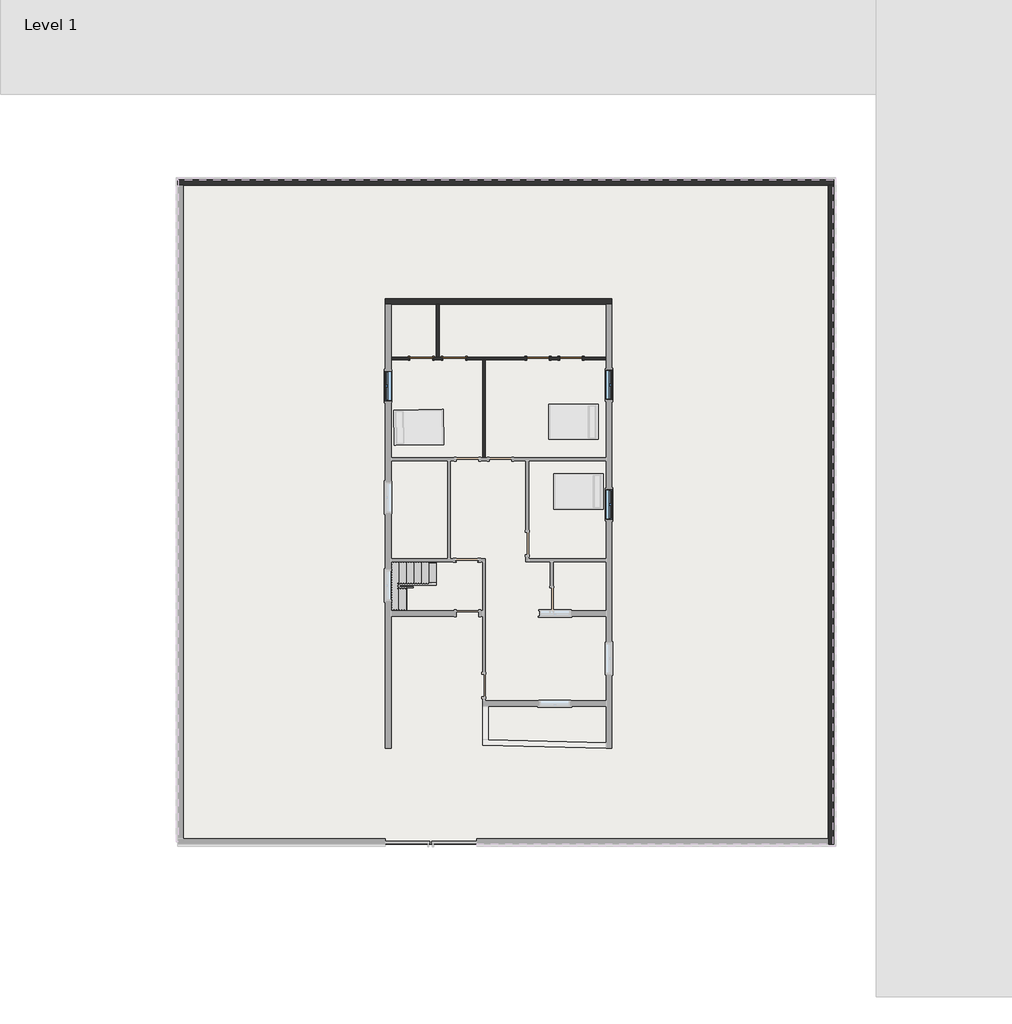
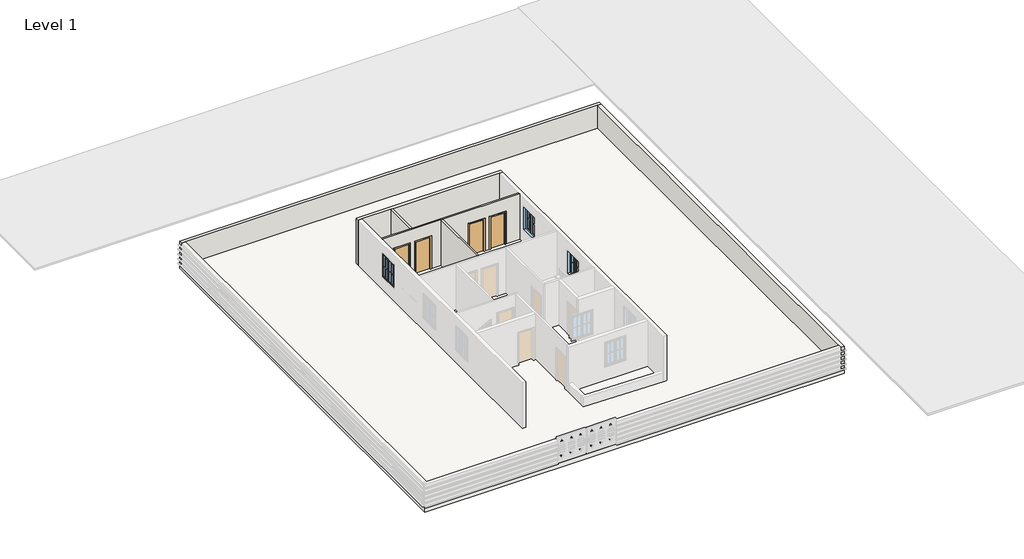
# One storey, part 2 of 3: 6 walls, 4 doors, 3 windows, 1 railing, 1 slab, 1 stair flight.
"""IFC4 building model written with IfcOpenShell, lengths in millimetres."""

from ifc_helpers import new_model, si_unit, frame, origin, origin_with_axes, place, context, project, spatial, polyline, outline, extrude, faceted_brep, transform, mapped, element, save
from components import door_e5f9f3c4, door_305aa2a5, stair_flight_da774960, window_8377141f

model = new_model("IFC4")

# Units and contexts
model_context = context("Model", 3, world=origin())
ifc_project = project(units=[si_unit("LENGTHUNIT", "METRE", prefix="MILLI")], contexts=[model_context])

# Site, building, storey
site = spatial("IfcSite", under=ifc_project)
building = spatial("IfcBuilding", under=site)
storey = spatial("IfcBuildingStorey", under=building, Name="Level 1", Elevation=0.0)

# Doors
placement = place(None, origin())
door_shape = door_e5f9f3c4(model_context)
element("IfcDoor", 1, ObjectType="Single-Flush : 36\" x 84\"", at=placement, inside=storey, context=model_context, shape_type="MappedRepresentation", body=[
    mapped(door_shape, transform((7442.2, 11550.65, 0.0), x_axis=(1.0, 0.0, 0.0), y_axis=(0.0, 1.0, 0.0), z_axis=(0.0, 0.0, 1.0))),
])
element("IfcDoor", 2, ObjectType="Single-Flush : 36\" x 84\"", at=placement, inside=storey, context=model_context, shape_type="MappedRepresentation", body=[
    mapped(door_shape, transform((2717.8, 11550.65, 0.0), x_axis=(1.0, 0.0, 0.0), y_axis=(0.0, 1.0, 0.0), z_axis=(0.0, 0.0, 1.0))),
])
door_2_shape = door_305aa2a5(model_context)
element("IfcDoor", 3, ObjectType="Single-Flush : 36\" x 84\"", at=placement, inside=storey, context=model_context, shape_type="MappedRepresentation", body=[
    mapped(door_2_shape, transform((4051.3, 11550.65, 0.0), x_axis=(-1.0, 0.0, 0.0), y_axis=(0.0, -1.0, 0.0), z_axis=(0.0, 0.0, 1.0))),
])
element("IfcDoor", 4, ObjectType="Single-Flush : 36\" x 84\"", at=placement, inside=storey, context=model_context, shape_type="MappedRepresentation", body=[
    mapped(door_2_shape, transform((8775.7, 11550.65, 0.0), x_axis=(-1.0, 0.0, 0.0), y_axis=(0.0, -1.0, 0.0), z_axis=(0.0, 0.0, 1.0))),
])

# Railing
element("IfcRailing", 5, ObjectType="Handrail - Rectangular", at=placement, inside=storey, context=model_context, shape_type="SolidModel", body=[
    faceted_brep([(3327.4, 3289.3, 1083.7333333), (3327.4, 3289.3, 1025.620221), (3327.4, 3340.1, 1025.620221), (3327.4, 3340.1, 1083.7333333), (1803.4, 3289.3, 1930.4), (1790.2363978, 3289.3, 1879.6), (1790.2363978, 3340.1, 1879.6), (1803.4, 3340.1, 1930.4), (1549.4, 3289.3, 1930.4), (1549.4, 3289.3, 1879.6), (1498.6, 3340.1, 1879.6), (1498.6, 3340.1, 1930.4), (1549.4, 1485.9, 1930.4), (1549.4, 1435.1, 1879.6), (1498.6, 1435.1, 1879.6), (1498.6, 1485.9, 1930.4), (1549.4, 1485.9, 2000.9555556), (1549.4, 1435.1, 1950.1555556), (1498.6, 1435.1, 1950.1555556), (1498.6, 1485.9, 2000.9555556), (1549.4, 1409.7, 2000.9555556), (1549.4, 1409.7, 1950.1555556), (1498.6, 1358.9, 1950.1555556), (1498.6, 1358.9, 2000.9555556), (1625.6, 1409.7, 2000.9555556), (1638.7636022, 1409.7, 1950.1555556), (1638.7636022, 1358.9, 1950.1555556), (1625.6, 1358.9, 2000.9555556), (3022.6, 1409.7, 2777.0666667), (3022.6, 1358.9, 2777.0666667), (3022.6, 1358.9, 2718.9535543), (3022.6, 1409.7, 2718.9535543)], [[[0, 1, 2, 3]], [[1, 0, 4, 5]], [[2, 1, 5, 6]], [[3, 2, 6, 7]], [[0, 3, 7, 4]], [[5, 4, 8, 9]], [[6, 5, 9, 10]], [[7, 6, 10, 11]], [[4, 7, 11, 8]], [[9, 8, 12, 13]], [[10, 9, 13, 14]], [[11, 10, 14, 15]], [[8, 11, 15, 12]], [[13, 12, 16, 17]], [[14, 13, 17, 18]], [[15, 14, 18, 19]], [[12, 15, 19, 16]], [[17, 16, 20, 21]], [[18, 17, 21, 22]], [[19, 18, 22, 23]], [[16, 19, 23, 20]], [[21, 20, 24, 25]], [[22, 21, 25, 26]], [[23, 22, 26, 27]], [[20, 23, 27, 24]], [[28, 29, 30, 31]], [[25, 24, 28, 31]], [[26, 25, 31, 30]], [[27, 26, 30, 29]], [[24, 27, 29, 28]]]),
    extrude(outline(polyline([(2681.9118876, 2955.925), (2671.3285543, 2936.875), (1693.3333333, 2936.875), (1693.3333333, 2955.925), (2681.9118876, 2955.925)])), frame((0.0, 1374.775, 0.0), z_axis=(0.0, 1.0, 0.0), x_axis=(0.0, 0.0, 1.0)), (0.0, 0.0, 1.0), 19.05),
    extrude(outline(polyline([(2625.4674432, 2854.325), (2614.8841099, 2835.275), (1693.3333333, 2835.275), (1693.3333333, 2854.325), (2625.4674432, 2854.325)])), frame((0.0, 1374.775, 0.0), z_axis=(0.0, 1.0, 0.0), x_axis=(0.0, 0.0, 1.0)), (0.0, 0.0, 1.0), 19.05),
    extrude(outline(polyline([(2569.0229988, 2752.725), (2558.4396654, 2733.675), (1693.3333333, 2733.675), (1693.3333333, 2752.725), (2569.0229988, 2752.725)])), frame((0.0, 1374.775, 0.0), z_axis=(0.0, 1.0, 0.0), x_axis=(0.0, 0.0, 1.0)), (0.0, 0.0, 1.0), 19.05),
    extrude(outline(polyline([(2512.5785543, 2651.125), (2501.995221, 2632.075), (1524.0, 2632.075), (1524.0, 2651.125), (2512.5785543, 2651.125)])), frame((0.0, 1374.775, 0.0), z_axis=(0.0, 1.0, 0.0), x_axis=(0.0, 0.0, 1.0)), (0.0, 0.0, 1.0), 19.05),
    extrude(outline(polyline([(2456.1341099, 2549.525), (2445.5507765, 2530.475), (1524.0, 2530.475), (1524.0, 2549.525), (2456.1341099, 2549.525)])), frame((0.0, 1374.775, 0.0), z_axis=(0.0, 1.0, 0.0), x_axis=(0.0, 0.0, 1.0)), (0.0, 0.0, 1.0), 19.05),
    extrude(outline(polyline([(2399.6896654, 2447.925), (2389.1063321, 2428.875), (1524.0, 2428.875), (1524.0, 2447.925), (2399.6896654, 2447.925)])), frame((0.0, 1374.775, 0.0), z_axis=(0.0, 1.0, 0.0), x_axis=(0.0, 0.0, 1.0)), (0.0, 0.0, 1.0), 19.05),
    extrude(outline(polyline([(2343.245221, 2346.325), (2332.6618876, 2327.275), (1354.6666667, 2327.275), (1354.6666667, 2346.325), (2343.245221, 2346.325)])), frame((0.0, 1374.775, 0.0), z_axis=(0.0, 1.0, 0.0), x_axis=(0.0, 0.0, 1.0)), (0.0, 0.0, 1.0), 19.05),
    extrude(outline(polyline([(2286.8007765, 2244.725), (2276.2174432, 2225.675), (1354.6666667, 2225.675), (1354.6666667, 2244.725), (2286.8007765, 2244.725)])), frame((0.0, 1374.775, 0.0), z_axis=(0.0, 1.0, 0.0), x_axis=(0.0, 0.0, 1.0)), (0.0, 0.0, 1.0), 19.05),
    extrude(outline(polyline([(2230.3563321, 2143.125), (2219.7729988, 2124.075), (1354.6666667, 2124.075), (1354.6666667, 2143.125), (2230.3563321, 2143.125)])), frame((0.0, 1374.775, 0.0), z_axis=(0.0, 1.0, 0.0), x_axis=(0.0, 0.0, 1.0)), (0.0, 0.0, 1.0), 19.05),
    extrude(outline(polyline([(2173.9118876, 2041.525), (2163.3285543, 2022.475), (1185.3333333, 2022.475), (1185.3333333, 2041.525), (2173.9118876, 2041.525)])), frame((0.0, 1374.775, 0.0), z_axis=(0.0, 1.0, 0.0), x_axis=(0.0, 0.0, 1.0)), (0.0, 0.0, 1.0), 19.05),
    extrude(outline(polyline([(2117.4674432, 1939.925), (2106.8841099, 1920.875), (1185.3333333, 1920.875), (1185.3333333, 1939.925), (2117.4674432, 1939.925)])), frame((0.0, 1374.775, 0.0), z_axis=(0.0, 1.0, 0.0), x_axis=(0.0, 0.0, 1.0)), (0.0, 0.0, 1.0), 19.05),
    extrude(outline(polyline([(2061.0229988, 1838.325), (2050.4396654, 1819.275), (1185.3333333, 1819.275), (1185.3333333, 1838.325), (2061.0229988, 1838.325)])), frame((0.0, 1374.775, 0.0), z_axis=(0.0, 1.0, 0.0), x_axis=(0.0, 0.0, 1.0)), (0.0, 0.0, 1.0), 19.05),
    extrude(outline(polyline([(2004.5785543, 1736.725), (1993.995221, 1717.675), (1016.0, 1717.675), (1016.0, 1736.725), (2004.5785543, 1736.725)])), frame((0.0, 1374.775, 0.0), z_axis=(0.0, 1.0, 0.0), x_axis=(0.0, 0.0, 1.0)), (0.0, 0.0, 1.0), 19.05),
    extrude(outline(polyline([(1948.1341099, 1635.125), (1937.5507765, 1616.075), (1016.0, 1616.075), (1016.0, 1635.125), (1948.1341099, 1635.125)])), frame((0.0, 1374.775, 0.0), z_axis=(0.0, 1.0, 0.0), x_axis=(0.0, 0.0, 1.0)), (0.0, 0.0, 1.0), 19.05),
    extrude(outline(polyline([(1514.475, 1495.425), (1533.525, 1495.425), (1533.525, 1476.375), (1514.475, 1476.375), (1514.475, 1495.425)])), frame((0.0, 0.0, 1016.0), z_axis=(0.0, 0.0, 1.0), x_axis=(1.0, 0.0, 0.0)), (0.0, 0.0, 1.0), 863.6),
    extrude(outline(polyline([(1514.475, 1597.025), (1533.525, 1597.025), (1533.525, 1577.975), (1514.475, 1577.975), (1514.475, 1597.025)])), frame((0.0, 0.0, 1016.0), z_axis=(0.0, 0.0, 1.0), x_axis=(1.0, 0.0, 0.0)), (0.0, 0.0, 1.0), 863.6),
    extrude(outline(polyline([(1514.475, 1698.625), (1533.525, 1698.625), (1533.525, 1679.575), (1514.475, 1679.575), (1514.475, 1698.625)])), frame((0.0, 0.0, 1016.0), z_axis=(0.0, 0.0, 1.0), x_axis=(1.0, 0.0, 0.0)), (0.0, 0.0, 1.0), 863.6),
    extrude(outline(polyline([(1514.475, 1800.225), (1533.525, 1800.225), (1533.525, 1781.175), (1514.475, 1781.175), (1514.475, 1800.225)])), frame((0.0, 0.0, 1016.0), z_axis=(0.0, 0.0, 1.0), x_axis=(1.0, 0.0, 0.0)), (0.0, 0.0, 1.0), 863.6),
    extrude(outline(polyline([(1514.475, 1901.825), (1533.525, 1901.825), (1533.525, 1882.775), (1514.475, 1882.775), (1514.475, 1901.825)])), frame((0.0, 0.0, 1016.0), z_axis=(0.0, 0.0, 1.0), x_axis=(1.0, 0.0, 0.0)), (0.0, 0.0, 1.0), 863.6),
    extrude(outline(polyline([(1514.475, 2003.425), (1533.525, 2003.425), (1533.525, 1984.375), (1514.475, 1984.375), (1514.475, 2003.425)])), frame((0.0, 0.0, 1016.0), z_axis=(0.0, 0.0, 1.0), x_axis=(1.0, 0.0, 0.0)), (0.0, 0.0, 1.0), 863.6),
    extrude(outline(polyline([(1514.475, 2105.025), (1533.525, 2105.025), (1533.525, 2085.975), (1514.475, 2085.975), (1514.475, 2105.025)])), frame((0.0, 0.0, 1016.0), z_axis=(0.0, 0.0, 1.0), x_axis=(1.0, 0.0, 0.0)), (0.0, 0.0, 1.0), 863.6),
    extrude(outline(polyline([(1514.475, 2206.625), (1533.525, 2206.625), (1533.525, 2187.575), (1514.475, 2187.575), (1514.475, 2206.625)])), frame((0.0, 0.0, 1016.0), z_axis=(0.0, 0.0, 1.0), x_axis=(1.0, 0.0, 0.0)), (0.0, 0.0, 1.0), 863.6),
    extrude(outline(polyline([(1514.475, 2308.225), (1533.525, 2308.225), (1533.525, 2289.175), (1514.475, 2289.175), (1514.475, 2308.225)])), frame((0.0, 0.0, 1016.0), z_axis=(0.0, 0.0, 1.0), x_axis=(1.0, 0.0, 0.0)), (0.0, 0.0, 1.0), 863.6),
    extrude(outline(polyline([(1514.475, 2409.825), (1533.525, 2409.825), (1533.525, 2390.775), (1514.475, 2390.775), (1514.475, 2409.825)])), frame((0.0, 0.0, 1016.0), z_axis=(0.0, 0.0, 1.0), x_axis=(1.0, 0.0, 0.0)), (0.0, 0.0, 1.0), 863.6),
    extrude(outline(polyline([(1514.475, 2511.425), (1533.525, 2511.425), (1533.525, 2492.375), (1514.475, 2492.375), (1514.475, 2511.425)])), frame((0.0, 0.0, 1016.0), z_axis=(0.0, 0.0, 1.0), x_axis=(1.0, 0.0, 0.0)), (0.0, 0.0, 1.0), 863.6),
    extrude(outline(polyline([(1514.475, 2613.025), (1533.525, 2613.025), (1533.525, 2593.975), (1514.475, 2593.975), (1514.475, 2613.025)])), frame((0.0, 0.0, 1016.0), z_axis=(0.0, 0.0, 1.0), x_axis=(1.0, 0.0, 0.0)), (0.0, 0.0, 1.0), 863.6),
    extrude(outline(polyline([(1514.475, 2714.625), (1533.525, 2714.625), (1533.525, 2695.575), (1514.475, 2695.575), (1514.475, 2714.625)])), frame((0.0, 0.0, 1016.0), z_axis=(0.0, 0.0, 1.0), x_axis=(1.0, 0.0, 0.0)), (0.0, 0.0, 1.0), 863.6),
    extrude(outline(polyline([(1514.475, 2816.225), (1533.525, 2816.225), (1533.525, 2797.175), (1514.475, 2797.175), (1514.475, 2816.225)])), frame((0.0, 0.0, 1016.0), z_axis=(0.0, 0.0, 1.0), x_axis=(1.0, 0.0, 0.0)), (0.0, 0.0, 1.0), 863.6),
    extrude(outline(polyline([(1514.475, 2917.825), (1533.525, 2917.825), (1533.525, 2898.775), (1514.475, 2898.775), (1514.475, 2917.825)])), frame((0.0, 0.0, 1016.0), z_axis=(0.0, 0.0, 1.0), x_axis=(1.0, 0.0, 0.0)), (0.0, 0.0, 1.0), 863.6),
    extrude(outline(polyline([(1514.475, 3019.425), (1533.525, 3019.425), (1533.525, 3000.375), (1514.475, 3000.375), (1514.475, 3019.425)])), frame((0.0, 0.0, 1016.0), z_axis=(0.0, 0.0, 1.0), x_axis=(1.0, 0.0, 0.0)), (0.0, 0.0, 1.0), 863.6),
    extrude(outline(polyline([(1514.475, 3121.025), (1533.525, 3121.025), (1533.525, 3101.975), (1514.475, 3101.975), (1514.475, 3121.025)])), frame((0.0, 0.0, 1016.0), z_axis=(0.0, 0.0, 1.0), x_axis=(1.0, 0.0, 0.0)), (0.0, 0.0, 1.0), 863.6),
    extrude(outline(polyline([(1514.475, 3222.625), (1533.525, 3222.625), (1533.525, 3203.575), (1514.475, 3203.575), (1514.475, 3222.625)])), frame((0.0, 0.0, 1016.0), z_axis=(0.0, 0.0, 1.0), x_axis=(1.0, 0.0, 0.0)), (0.0, 0.0, 1.0), 863.6),
    extrude(outline(polyline([(1609.725, 3324.225), (1609.725, 3305.175), (1590.675, 3305.175), (1590.675, 3324.225), (1609.725, 3324.225)])), frame((0.0, 0.0, 1016.0), z_axis=(0.0, 0.0, 1.0), x_axis=(1.0, 0.0, 0.0)), (0.0, 0.0, 1.0), 863.6),
    extrude(outline(polyline([(1711.325, 3324.225), (1711.325, 3305.175), (1692.275, 3305.175), (1692.275, 3324.225), (1711.325, 3324.225)])), frame((0.0, 0.0, 1016.0), z_axis=(0.0, 0.0, 1.0), x_axis=(1.0, 0.0, 0.0)), (0.0, 0.0, 1.0), 863.6),
    extrude(outline(polyline([(1866.995221, 1812.925), (1877.5785543, 1793.875), (1016.0, 1793.875), (1016.0, 1812.925), (1866.995221, 1812.925)])), frame((0.0, 3305.175, 0.0), z_axis=(0.0, 1.0, 0.0), x_axis=(0.0, 0.0, 1.0)), (0.0, 0.0, 1.0), 19.05),
    extrude(outline(polyline([(1810.5507765, 1914.525), (1821.1341099, 1895.475), (846.6666667, 1895.475), (846.6666667, 1914.525), (1810.5507765, 1914.525)])), frame((0.0, 3305.175, 0.0), z_axis=(0.0, 1.0, 0.0), x_axis=(0.0, 0.0, 1.0)), (0.0, 0.0, 1.0), 19.05),
    extrude(outline(polyline([(1754.1063321, 2016.125), (1764.6896654, 1997.075), (846.6666667, 1997.075), (846.6666667, 2016.125), (1754.1063321, 2016.125)])), frame((0.0, 3305.175, 0.0), z_axis=(0.0, 1.0, 0.0), x_axis=(0.0, 0.0, 1.0)), (0.0, 0.0, 1.0), 19.05),
    extrude(outline(polyline([(1697.6618876, 2117.725), (1708.245221, 2098.675), (846.6666667, 2098.675), (846.6666667, 2117.725), (1697.6618876, 2117.725)])), frame((0.0, 3305.175, 0.0), z_axis=(0.0, 1.0, 0.0), x_axis=(0.0, 0.0, 1.0)), (0.0, 0.0, 1.0), 19.05),
    extrude(outline(polyline([(1641.2174432, 2219.325), (1651.8007765, 2200.275), (677.3333333, 2200.275), (677.3333333, 2219.325), (1641.2174432, 2219.325)])), frame((0.0, 3305.175, 0.0), z_axis=(0.0, 1.0, 0.0), x_axis=(0.0, 0.0, 1.0)), (0.0, 0.0, 1.0), 19.05),
    extrude(outline(polyline([(1584.7729988, 2320.925), (1595.3563321, 2301.875), (677.3333333, 2301.875), (677.3333333, 2320.925), (1584.7729988, 2320.925)])), frame((0.0, 3305.175, 0.0), z_axis=(0.0, 1.0, 0.0), x_axis=(0.0, 0.0, 1.0)), (0.0, 0.0, 1.0), 19.05),
    extrude(outline(polyline([(1528.3285543, 2422.525), (1538.9118876, 2403.475), (677.3333333, 2403.475), (677.3333333, 2422.525), (1528.3285543, 2422.525)])), frame((0.0, 3305.175, 0.0), z_axis=(0.0, 1.0, 0.0), x_axis=(0.0, 0.0, 1.0)), (0.0, 0.0, 1.0), 19.05),
    extrude(outline(polyline([(1471.8841099, 2524.125), (1482.4674432, 2505.075), (508.0, 2505.075), (508.0, 2524.125), (1471.8841099, 2524.125)])), frame((0.0, 3305.175, 0.0), z_axis=(0.0, 1.0, 0.0), x_axis=(0.0, 0.0, 1.0)), (0.0, 0.0, 1.0), 19.05),
    extrude(outline(polyline([(1415.4396654, 2625.725), (1426.0229988, 2606.675), (508.0, 2606.675), (508.0, 2625.725), (1415.4396654, 2625.725)])), frame((0.0, 3305.175, 0.0), z_axis=(0.0, 1.0, 0.0), x_axis=(0.0, 0.0, 1.0)), (0.0, 0.0, 1.0), 19.05),
    extrude(outline(polyline([(1358.995221, 2727.325), (1369.5785543, 2708.275), (508.0, 2708.275), (508.0, 2727.325), (1358.995221, 2727.325)])), frame((0.0, 3305.175, 0.0), z_axis=(0.0, 1.0, 0.0), x_axis=(0.0, 0.0, 1.0)), (0.0, 0.0, 1.0), 19.05),
    extrude(outline(polyline([(1302.5507765, 2828.925), (1313.1341099, 2809.875), (338.6666667, 2809.875), (338.6666667, 2828.925), (1302.5507765, 2828.925)])), frame((0.0, 3305.175, 0.0), z_axis=(0.0, 1.0, 0.0), x_axis=(0.0, 0.0, 1.0)), (0.0, 0.0, 1.0), 19.05),
    extrude(outline(polyline([(1246.1063321, 2930.525), (1256.6896654, 2911.475), (338.6666667, 2911.475), (338.6666667, 2930.525), (1246.1063321, 2930.525)])), frame((0.0, 3305.175, 0.0), z_axis=(0.0, 1.0, 0.0), x_axis=(0.0, 0.0, 1.0)), (0.0, 0.0, 1.0), 19.05),
    extrude(outline(polyline([(1189.6618876, 3032.125), (1200.245221, 3013.075), (338.6666667, 3013.075), (338.6666667, 3032.125), (1189.6618876, 3032.125)])), frame((0.0, 3305.175, 0.0), z_axis=(0.0, 1.0, 0.0), x_axis=(0.0, 0.0, 1.0)), (0.0, 0.0, 1.0), 19.05),
    extrude(outline(polyline([(1133.2174432, 3133.725), (1143.8007765, 3114.675), (169.3333333, 3114.675), (169.3333333, 3133.725), (1133.2174432, 3133.725)])), frame((0.0, 3305.175, 0.0), z_axis=(0.0, 1.0, 0.0), x_axis=(0.0, 0.0, 1.0)), (0.0, 0.0, 1.0), 19.05),
    extrude(outline(polyline([(1076.7729988, 3235.325), (1087.3563321, 3216.275), (169.3333333, 3216.275), (169.3333333, 3235.325), (1076.7729988, 3235.325)])), frame((0.0, 3305.175, 0.0), z_axis=(0.0, 1.0, 0.0), x_axis=(0.0, 0.0, 1.0)), (0.0, 0.0, 1.0), 19.05),
    extrude(outline(polyline([(1514.475, 1393.825), (1533.525, 1393.825), (1533.525, 1374.775), (1514.475, 1374.775), (1514.475, 1393.825)])), frame((0.0, 0.0, 1016.0), z_axis=(0.0, 0.0, 1.0), x_axis=(1.0, 0.0, 0.0)), (0.0, 0.0, 1.0), 934.1555556),
    extrude(outline(polyline([(1533.525, 3324.225), (1533.525, 3305.175), (1514.475, 3305.175), (1514.475, 3324.225), (1533.525, 3324.225)])), frame((0.0, 0.0, 1016.0), z_axis=(0.0, 0.0, 1.0), x_axis=(1.0, 0.0, 0.0)), (0.0, 0.0, 1.0), 863.6),
    extrude(outline(polyline([(2718.9535543, 3022.6), (2708.370221, 3003.55), (1693.3333333, 3003.55), (1693.3333333, 3022.6), (2718.9535543, 3022.6)])), frame((0.0, 1374.775, 0.0), z_axis=(0.0, 1.0, 0.0), x_axis=(0.0, 0.0, 1.0)), (0.0, 0.0, 1.0), 19.05),
    extrude(outline(polyline([(1025.620221, 3327.4), (1036.2035543, 3308.35), (169.3333333, 3308.35), (169.3333333, 3327.4), (1025.620221, 3327.4)])), frame((0.0, 3305.175, 0.0), z_axis=(0.0, 1.0, 0.0), x_axis=(0.0, 0.0, 1.0)), (0.0, 0.0, 1.0), 19.05),
])

# Slab
element("IfcSlab", 6, ObjectType="Generic - 12\"", at=placement, inside=storey, context=model_context, shape_type="SweptSolid", body=[
    extrude(outline(polyline([(19396.129742, 18780.9634228), (19396.129742, -8092.2365772), (-7121.470258, -8092.2365772), (-7121.470258, 18780.9634228), (19396.129742, 18780.9634228)])), frame((0.0, 0.0, -304.8), z_axis=(0.0, 0.0, 1.0), x_axis=(1.0, 0.0, 0.0)), (0.0, 0.0, 1.0), 304.8),
])

# Stair flight
stair_flight_shape = stair_flight_da774960(model_context)
element("IfcStairFlight", 7, ObjectType="2\" Tread 1\" Nosing 1/4\" Riser", at=placement, inside=storey, context=model_context, shape_type="MappedRepresentation", body=[
    mapped(stair_flight_shape, transform((0.0, 0.0, 0.0), x_axis=(1.0, 0.0, 0.0), y_axis=(0.0, 1.0, 0.0), z_axis=(0.0, 0.0, 1.0))),
])

# Walls
element("IfcWall", 8, ObjectType="Generic - 5\"", at=placement, inside=storey, context=model_context, shape_type="SweptSolid", body=[
    extrude(outline(polyline([(3327.4, 11607.8), (3327.4, 13741.4), (3441.7, 13741.4), (3441.7, 11607.8), (3327.4, 11607.8)])), origin_with_axes(), (0.0, 0.0, 1.0), 3048.0),
])
element("IfcWall", 9, ObjectType="Generic - 5\"", at=placement, inside=storey, context=model_context, shape_type="Brep", body=[
    faceted_brep([(7899.4, 11493.5, 0.0), (8318.5, 11493.5, 0.0), (8318.5, 11493.5, 2133.6), (9232.9, 11493.5, 2133.6), (9232.9, 11493.5, 0.0), (10185.4, 11493.5, 0.0), (10185.4, 11493.5, 3048.0), (5308.6, 11493.5, 3048.0), (5194.3, 11493.5, 3048.0), (1498.6, 11493.5, 3048.0), (1498.6, 11493.5, 0.0), (2260.6, 11493.5, 0.0), (2260.6, 11493.5, 2133.6), (3175.0, 11493.5, 2133.6), (3175.0, 11493.5, 0.0), (3594.1, 11493.5, 0.0), (3594.1, 11493.5, 2133.6), (4508.5, 11493.5, 2133.6), (4508.5, 11493.5, 0.0), (5194.3, 11493.5, 0.0), (5308.6, 11493.5, 0.0), (6985.0, 11493.5, 0.0), (6985.0, 11493.5, 2133.6), (7899.4, 11493.5, 2133.6), (8318.5, 11607.8, 2133.6), (8318.5, 11607.8, 0.0), (7899.4, 11607.8, 0.0), (7899.4, 11607.8, 2133.6), (6985.0, 11607.8, 2133.6), (6985.0, 11607.8, 0.0), (4508.5, 11607.8, 0.0), (4508.5, 11607.8, 2133.6), (3594.1, 11607.8, 2133.6), (3594.1, 11607.8, 0.0), (3441.7, 11607.8, 0.0), (3327.4, 11607.8, 0.0), (3175.0, 11607.8, 0.0), (3175.0, 11607.8, 2133.6), (2260.6, 11607.8, 2133.6), (2260.6, 11607.8, 0.0), (1498.6, 11607.8, 0.0), (1498.6, 11607.8, 3048.0), (3327.4, 11607.8, 3048.0), (3441.7, 11607.8, 3048.0), (10185.4, 11607.8, 3048.0), (10185.4, 11607.8, 0.0), (9232.9, 11607.8, 0.0), (9232.9, 11607.8, 2133.6)], [[[0, 1, 2, 3, 4, 5, 6, 7, 8, 9, 10, 11, 12, 13, 14, 15, 16, 17, 18, 19, 20, 21, 22, 23]], [[24, 25, 26, 27, 28, 29, 30, 31, 32, 33, 34, 35, 36, 37, 38, 39, 40, 41, 42, 43, 44, 45, 46, 47]], [[11, 10, 40, 39]], [[30, 29, 21, 20, 19, 18]], [[36, 35, 34, 33, 15, 14]], [[46, 45, 5, 4]], [[26, 25, 1, 0]], [[9, 8, 7, 6, 44, 43, 42, 41]], [[6, 5, 45, 44]], [[10, 9, 41, 40]], [[27, 26, 0, 23]], [[28, 27, 23, 22]], [[29, 28, 22, 21]], [[37, 36, 14, 13]], [[38, 37, 13, 12]], [[39, 38, 12, 11]], [[16, 15, 33, 32]], [[17, 16, 32, 31]], [[18, 17, 31, 30]], [[2, 1, 25, 24]], [[3, 2, 24, 47]], [[4, 3, 47, 46]]]),
])
element("IfcWall", 10, ObjectType="Generic - 5\"", at=placement, inside=storey, context=model_context, shape_type="SweptSolid", body=[
    extrude(outline(polyline([(5194.3, 7531.1), (5194.3, 11493.5), (5308.6, 11493.5), (5308.6, 7531.1), (5194.3, 7531.1)])), origin_with_axes(), (0.0, 0.0, 1.0), 3048.0),
])
element("IfcWall", 11, ObjectType="Generic - 8\"", at=placement, inside=storey, context=model_context, shape_type="Brep", body=[
    faceted_brep([(1270.0, 13741.4, 0.0), (1498.6, 13741.4, 0.0), (3327.4, 13741.4, 0.0), (3441.7, 13741.4, 0.0), (10185.4, 13741.4, 0.0), (10414.0, 13741.4, 0.0), (10414.0, 13741.4, 3048.0), (10185.4, 13741.4, 3048.0), (3441.7, 13741.4, 3048.0), (3327.4, 13741.4, 3048.0), (1498.6, 13741.4, 3048.0), (1270.0, 13741.4, 3048.0), (1270.0, 13970.0, 0.0), (1270.0, 13970.0, 3048.0), (10414.0, 13970.0, 3048.0), (10414.0, 13970.0, 0.0)], [[[0, 1, 2, 3, 4, 5, 6, 7, 8, 9, 10, 11]], [[12, 13, 14, 15]], [[5, 4, 3, 2, 1, 0, 12, 15]], [[6, 5, 15, 14]], [[0, 11, 13, 12]], [[11, 10, 9, 8, 7, 6, 14, 13]]]),
])
element("IfcWall", 12, ObjectType="Generic - 8\"", at=placement, inside=storey, context=model_context, shape_type="Brep", body=[
    faceted_brep([(19396.129742, 18552.3634228, 1524.0), (19167.529742, 18552.3634228, 1524.0), (-6892.870258, 18552.3634228, 1524.0), (-7121.470258, 18552.3634228, 1524.0), (-7121.470258, 18552.3634228, 1337.7333333), (-7096.070258, 18552.3634228, 1337.7333333), (-7096.070258, 18552.3634228, 1270.0), (-7121.470258, 18552.3634228, 1270.0), (-7121.470258, 18552.3634228, 1032.9333333), (-7096.070258, 18552.3634228, 1032.9333333), (-7096.070258, 18552.3634228, 914.4), (-7121.470258, 18552.3634228, 914.4), (-7121.470258, 18552.3634228, 677.3333333), (-7096.070258, 18552.3634228, 677.3333333), (-7096.070258, 18552.3634228, 609.6), (-7121.470258, 18552.3634228, 609.6), (-7121.470258, 18552.3634228, 372.5333333), (-7096.070258, 18552.3634228, 372.5333333), (-7096.070258, 18552.3634228, 304.8), (-7121.470258, 18552.3634228, 304.8), (-7121.470258, 18552.3634228, 67.7333333), (-7096.070258, 18552.3634228, 67.7333333), (-7096.070258, 18552.3634228, 0.0), (-6892.870258, 18552.3634228, 0.0), (19167.529742, 18552.3634228, 0.0), (19370.729742, 18552.3634228, 0.0), (19370.729742, 18552.3634228, 67.7333333), (19396.129742, 18552.3634228, 67.7333333), (19396.129742, 18552.3634228, 304.8), (19370.729742, 18552.3634228, 304.8), (19370.729742, 18552.3634228, 372.5333333), (19396.129742, 18552.3634228, 372.5333333), (19396.129742, 18552.3634228, 609.6), (19370.729742, 18552.3634228, 609.6), (19370.729742, 18552.3634228, 677.3333333), (19396.129742, 18552.3634228, 677.3333333), (19396.129742, 18552.3634228, 914.4), (19370.729742, 18552.3634228, 914.4), (19370.729742, 18552.3634228, 982.1333333), (19396.129742, 18552.3634228, 982.1333333), (19396.129742, 18552.3634228, 1219.2), (19370.729742, 18552.3634228, 1219.2), (19370.729742, 18552.3634228, 1286.9333333), (19396.129742, 18552.3634228, 1286.9333333), (-7121.470258, 18780.9634228, 1524.0), (19396.129742, 18780.9634228, 1524.0), (19396.129742, 18780.9634228, 1286.9333333), (-7096.070258, 18780.9634228, 1286.9333333), (-7096.070258, 18780.9634228, 1337.7333333), (-7121.470258, 18780.9634228, 1337.7333333), (19396.129742, 18780.9634228, 67.7333333), (-7121.470258, 18780.9634228, 67.7333333), (-7121.470258, 18780.9634228, 304.8), (19396.129742, 18780.9634228, 304.8), (19396.129742, 18780.9634228, 609.6), (19396.129742, 18780.9634228, 372.5333333), (-7121.470258, 18780.9634228, 372.5333333), (-7121.470258, 18780.9634228, 609.6), (19396.129742, 18780.9634228, 914.4), (19396.129742, 18780.9634228, 677.3333333), (-7121.470258, 18780.9634228, 677.3333333), (-7121.470258, 18780.9634228, 914.4), (19396.129742, 18780.9634228, 1219.2), (19396.129742, 18780.9634228, 982.1333333), (-7096.070258, 18780.9634228, 982.1333333), (-7096.070258, 18780.9634228, 1032.9333333), (-7121.470258, 18780.9634228, 1032.9333333), (-7121.470258, 18780.9634228, 1219.2), (-7096.070258, 18755.5634228, 0.0), (19370.729742, 18755.5634228, 0.0), (-7121.470258, 18755.5634228, 1219.2), (-7121.470258, 18755.5634228, 1270.0), (-7096.070258, 18755.5634228, 67.7333333), (19370.729742, 18755.5634228, 67.7333333), (-7096.070258, 18755.5634228, 304.8), (-7096.070258, 18755.5634228, 372.5333333), (19370.729742, 18755.5634228, 372.5333333), (19370.729742, 18755.5634228, 304.8), (-7096.070258, 18755.5634228, 609.6), (-7096.070258, 18755.5634228, 677.3333333), (19370.729742, 18755.5634228, 677.3333333), (19370.729742, 18755.5634228, 609.6), (-7096.070258, 18755.5634228, 982.1333333), (19370.729742, 18755.5634228, 982.1333333), (19370.729742, 18755.5634228, 914.4), (-7096.070258, 18755.5634228, 914.4), (19370.729742, 18755.5634228, 1286.9333333), (-7096.070258, 18755.5634228, 1286.9333333), (19370.729742, 18755.5634228, 1219.2), (-7096.070258, 18755.5634228, 1270.0)], [[[0, 1, 2, 3, 4, 5, 6, 7, 8, 9, 10, 11, 12, 13, 14, 15, 16, 17, 18, 19, 20, 21, 22, 23, 24, 25, 26, 27, 28, 29, 30, 31, 32, 33, 34, 35, 36, 37, 38, 39, 40, 41, 42, 43]], [[44, 45, 46, 47, 48, 49]], [[50, 51, 52, 53]], [[54, 55, 56, 57]], [[58, 59, 60, 61]], [[62, 63, 64, 65, 66, 67]], [[68, 69, 25, 24, 23, 22]], [[3, 2, 1, 0, 45, 44]], [[45, 0, 43, 46]], [[27, 50, 53, 28]], [[32, 31, 55, 54]], [[36, 35, 59, 58]], [[40, 39, 63, 62]], [[3, 44, 49, 4]], [[51, 20, 19, 52]], [[57, 56, 16, 15]], [[61, 60, 12, 11]], [[70, 67, 66, 8, 7, 71]], [[68, 72, 73, 69]], [[69, 73, 26, 25]], [[73, 72, 21, 20, 51, 50, 27, 26]], [[72, 68, 22, 21]], [[74, 75, 76, 77]], [[77, 76, 30, 29]], [[78, 79, 80, 81]], [[81, 80, 34, 33]], [[82, 83, 84, 85]], [[84, 83, 38, 37]], [[42, 86, 87, 47, 46, 43]], [[70, 88, 41, 40, 62, 67]], [[88, 70, 71, 89, 87, 86]], [[88, 86, 42, 41]], [[76, 75, 17, 16, 56, 55, 31, 30]], [[74, 77, 29, 28, 53, 52, 19, 18]], [[75, 74, 18, 17]], [[80, 79, 13, 12, 60, 59, 35, 34]], [[78, 81, 33, 32, 54, 57, 15, 14]], [[79, 78, 14, 13]], [[83, 82, 64, 63, 39, 38]], [[85, 84, 37, 36, 58, 61, 11, 10]], [[85, 10, 9, 65, 64, 82]], [[65, 9, 8, 66]], [[48, 5, 4, 49]], [[6, 89, 71, 7]], [[5, 48, 47, 87, 89, 6]]]),
])
element("IfcWall", 13, ObjectType="Generic - 8\"", at=placement, inside=storey, context=model_context, shape_type="Brep", body=[
    faceted_brep([(19167.529742, -8092.2365772, 1524.0), (19167.529742, -7863.6365772, 1524.0), (19167.529742, 18552.3634228, 1524.0), (19167.529742, 18552.3634228, 0.0), (19167.529742, -7863.6365772, 0.0), (19167.529742, -8066.8365772, 0.0), (19167.529742, -8066.8365772, 67.7333333), (19167.529742, -8092.2365772, 67.7333333), (19167.529742, -8092.2365772, 304.8), (19167.529742, -8066.8365772, 304.8), (19167.529742, -8066.8365772, 372.5333333), (19167.529742, -8092.2365772, 372.5333333), (19167.529742, -8092.2365772, 609.6), (19167.529742, -8066.8365772, 609.6), (19167.529742, -8066.8365772, 677.3333333), (19167.529742, -8092.2365772, 677.3333333), (19167.529742, -8092.2365772, 914.4), (19167.529742, -8066.8365772, 914.4), (19167.529742, -8066.8365772, 982.1333333), (19167.529742, -8092.2365772, 982.1333333), (19167.529742, -8092.2365772, 1219.2), (19167.529742, -8066.8365772, 1219.2), (19167.529742, -8066.8365772, 1286.9333333), (19167.529742, -8092.2365772, 1286.9333333), (19396.129742, 18552.3634228, 1524.0), (19396.129742, -8092.2365772, 1524.0), (19396.129742, -8092.2365772, 1286.9333333), (19396.129742, 18552.3634228, 1286.9333333), (19396.129742, -8092.2365772, 67.7333333), (19396.129742, 18552.3634228, 67.7333333), (19396.129742, 18552.3634228, 304.8), (19396.129742, -8092.2365772, 304.8), (19396.129742, -8092.2365772, 372.5333333), (19396.129742, 18552.3634228, 372.5333333), (19396.129742, 18552.3634228, 609.6), (19396.129742, -8092.2365772, 609.6), (19396.129742, -8092.2365772, 677.3333333), (19396.129742, 18552.3634228, 677.3333333), (19396.129742, 18552.3634228, 914.4), (19396.129742, -8092.2365772, 914.4), (19396.129742, -8092.2365772, 982.1333333), (19396.129742, 18552.3634228, 982.1333333), (19396.129742, 18552.3634228, 1219.2), (19396.129742, -8092.2365772, 1219.2), (19370.729742, 18552.3634228, 0.0), (19370.729742, -8066.8365772, 0.0), (19370.729742, 18552.3634228, 1286.9333333), (19370.729742, 18552.3634228, 1219.2), (19370.729742, 18552.3634228, 982.1333333), (19370.729742, 18552.3634228, 914.4), (19370.729742, 18552.3634228, 677.3333333), (19370.729742, 18552.3634228, 609.6), (19370.729742, 18552.3634228, 372.5333333), (19370.729742, 18552.3634228, 304.8), (19370.729742, 18552.3634228, 67.7333333), (19370.729742, -8066.8365772, 67.7333333), (19370.729742, -8066.8365772, 372.5333333), (19370.729742, -8066.8365772, 304.8), (19370.729742, -8066.8365772, 677.3333333), (19370.729742, -8066.8365772, 609.6), (19370.729742, -8066.8365772, 982.1333333), (19370.729742, -8066.8365772, 914.4), (19370.729742, -8066.8365772, 1286.9333333), (19370.729742, -8066.8365772, 1219.2)], [[[0, 1, 2, 3, 4, 5, 6, 7, 8, 9, 10, 11, 12, 13, 14, 15, 16, 17, 18, 19, 20, 21, 22, 23]], [[24, 25, 26, 27]], [[28, 29, 30, 31]], [[32, 33, 34, 35]], [[36, 37, 38, 39]], [[40, 41, 42, 43]], [[5, 4, 3, 44, 45]], [[2, 1, 0, 25, 24]], [[3, 2, 24, 27, 46, 47, 42, 41, 48, 49, 38, 37, 50, 51, 34, 33, 52, 53, 30, 29, 54, 44]], [[25, 0, 23, 26]], [[7, 28, 31, 8]], [[11, 32, 35, 12]], [[15, 36, 39, 16]], [[19, 40, 43, 20]], [[6, 55, 54, 29, 28, 7]], [[55, 45, 44, 54]], [[45, 55, 6, 5]], [[10, 56, 52, 33, 32, 11]], [[53, 57, 9, 8, 31, 30]], [[56, 57, 53, 52]], [[57, 56, 10, 9]], [[14, 58, 50, 37, 36, 15]], [[51, 59, 13, 12, 35, 34]], [[58, 59, 51, 50]], [[59, 58, 14, 13]], [[18, 60, 48, 41, 40, 19]], [[49, 61, 17, 16, 39, 38]], [[60, 61, 49, 48]], [[61, 60, 18, 17]], [[22, 62, 46, 27, 26, 23]], [[47, 63, 21, 20, 43, 42]], [[62, 63, 47, 46]], [[63, 62, 22, 21]]]),
])

# Windows
window_shape = window_8377141f(model_context)
element("IfcWindow", 14, ObjectType="Window-Casement-Double : 48\" x 60\"", at=placement, inside=storey, context=model_context, shape_type="MappedRepresentation", body=[
    mapped(window_shape, transform((1384.3, 10433.05, 0.0), x_axis=(0.0, 1.0, 0.0), y_axis=(-1.0, 0.0, 0.0), z_axis=(0.0, 0.0, 1.0))),
])
element("IfcWindow", 15, ObjectType="Window-Casement-Double : 48\" x 60\"", at=placement, inside=storey, context=model_context, shape_type="MappedRepresentation", body=[
    mapped(window_shape, transform((10299.7, 10483.85, 0.0), x_axis=(0.0, -1.0, 0.0), y_axis=(1.0, 0.0, 0.0), z_axis=(0.0, 0.0, 1.0))),
])
element("IfcWindow", 16, ObjectType="Window-Casement-Double : 48\" x 60\"", at=placement, inside=storey, context=model_context, shape_type="MappedRepresentation", body=[
    mapped(window_shape, transform((10299.7, 5645.15, 0.0), x_axis=(0.0, -1.0, 0.0), y_axis=(1.0, 0.0, 0.0), z_axis=(0.0, 0.0, 1.0))),
])

save(model, "model.ifc")

# Revit data of these elements
# Type "Single-Flush : 36\" x 84\""
#   Type Mark = "1"
#   Construction Type Id = "MDOOR"
#   Assembly Code = "C1020"
#   Analytic Construction = "Metal"
#   Thickness = 0' - 2"
#   Heat Transfer Coefficient (U) = 0.651978 BTU/(h·ft²·°F)
#   Height = 7' - 0"
#   Trim Projection Ext = 0' - 1"
#   Trim Projection Int = 0' - 1"
#   Trim Width = 0' - 3"
#   Width = 3' - 0"
#   Define Thermal Properties by = 1
#   Define Thermal Properties by = 1
#   Door Material = Door - Panel
#   Frame Material = Door - Frame
#   Visual Light Transmittance = 0
#   Solar Heat Gain Coefficient = 0
#   Function = (empty or 0)
#   Wall Closure = (empty or 0)
# Type "Handrail - Rectangular"
#   Assembly Code = "C2010400"
#   built-in parameter 1008612 = 0.0416667 (stored number, unit not read)
#   built-in parameter 1008611 = 0.0416667 (stored number, unit not read)
#   built-in parameter 1008609 = 0.333333 (stored number, unit not read)
#   built-in parameter 1008604 = 0.166667 (stored number, unit not read)
#   built-in parameter 1008603 = 0.166667 (stored number, unit not read)
#   Railing Height = 3' - 0"
#   built-in parameter 1008630 = 2
#   built-in parameter 1008610 = 2
#   built-in parameter 1008618 = Baluster - Square : 3/4"
# Type "Generic - 12\""
#   Assembly Code = "B1010"
#   Function = 0
#   Layers, outside or top first: 1' - 0" no material (function 1)
# Type "Generic - 5\""
#   Assembly Code = "B2010"
#   Layers, outside or top first: 0' - 4 1/2" no material (function 1)
# Type "Generic - 8\""
#   Assembly Code = "B2010"
# Type "Window-Casement-Double : 48\" x 60\""
#   Type Mark = "17"
#   Fire Rating = "0.5h"
#   Assembly Code = "B2020100"
#   Analytic Construction = "Double glazing - domestic"
#   Frame Extension [instance default] = 0' - 0 1/4"
#   Window Inset [instance default] = 0' - 0"
#   Wall Thickness [instance default] = 0' - 6"
#   Interior Wall Closure [instance default] = 0' - 2 1/4"
#   Half Width = 2' - 0"
#   Visual Light Transmittance = 0.81
#   Thermal Resistance (R) = 1.8146 (h·ft²·°F)/BTU
#   Solar Heat Gain Coefficient = 0.76
#   Rough Width = 4' - 0 1/2"
#   Rough Height = 5' - 0 1/2"
#   Height = 5' - 0"
#   Heat Transfer Coefficient (U) = 0.5511 BTU/(h·ft²·°F)
#   Exterior Wall Closure [instance default] = 0' - 1 1/4"
#   Extension Jamb [instance default] = 0' - 2 1/4"
#   Default Sill Height = 3' - 0"
#   Width = 4' - 0"
#   Define Thermal Properties by = 0
#   Muntin Visibility = yes
#   Interior Trim Visibility [instance default] = yes
#   Exterior Trim Visibility [instance default] = yes
#   Extension Jamb Visibility [instance default] = yes
#   Interior Trim Material = Wood - Stained
#   Muntin Pattern = Muntin Pattern_2x2 : Muntin Pattern_2x2
#   Interior Trim = Trim-Window-Interior-Flat : Picture Frame
#   Interior Frame Material = Wood - Stained
#   Glass Panel Material = Glass
#   Exterior Trim Material = Clad - White
#   Exterior Trim = Trim-Window-Exterior-Flat : with Sill
#   Exterior Frame Material = Clad - White
#   Wall Closure = (empty or 0)
# Elements 1, 2, 3, 4 (IfcDoor, "Single-Flush : 36\" x 84\"")
#   Phase Created = New Construction
#   Materials on its faces: "Door - Frame", "Door - Panel"
# Element 5 (IfcRailing, "Handrail - Rectangular")
#   Phase Created = New Construction
# Element 6 (IfcSlab, "Generic - 12\"")
#   Height Offset From Level = 0' - 0"
#   Phase Created = New Construction
#   Materials on its faces: "Clad - White", "Default Floor", "Wood Planks"
# Element 7 (IfcStairFlight, "2\" Tread 1\" Nosing 1/4\" Riser")
#   Phase Created = New Construction
# Elements 8, 9, 10 (IfcWall, "Generic - 5\"")
#   Top Offset = 0' - 0"
#   Base Offset = 0' - 0"
#   wall height = 10' - 0"
#   Phase Created = New Construction
#   Base Constraint = Level 1
#   Top Constraint = Level 2
#   Materials on its faces: "Default Wall"
# Element 11 (IfcWall, "Generic - 8\"")
#   Top Offset = 0' - 0"
#   Base Offset = 0' - 0"
#   Unconnected Height = 10' - 0"
#   wall height = 10' - 0"
#   Phase Created = New Construction
#   Base Constraint = Level 1
#   Materials on its faces: "Parking Stripe"
# Elements 12, 13 (IfcWall, "Generic - 8\"")
#   Top Offset = 0' - 0"
#   Base Offset = 0' - 0"
#   Unconnected Height = 5' - 0"
#   wall height = 5' - 0"
#   Phase Created = New Construction
#   Base Constraint = Level 1
#   Materials on its faces: "Clad - White"
# Element 14 (IfcWindow, "Window-Casement-Double : 48\" x 60\"")
#   Mark = "2"
#   Window Inset = 0' - 0"
#   Interior Wall Closure = 0' - 2 1/4"
#   Frame Extension = 0' - 0 1/4"
#   Exterior Wall Closure = 0' - 1 1/4"
#   Interior Trim Visibility = yes
#   Exterior Trim Visibility = yes
#   Phase Created = New Construction
#   Materials on its faces: "Wood - Stained", "Glass", "Clad - White"
# Element 15 (IfcWindow, "Window-Casement-Double : 48\" x 60\"")
#   Mark = "3"
#   Window Inset = 0' - 0"
#   Interior Wall Closure = 0' - 2 1/4"
#   Frame Extension = 0' - 0 1/4"
#   Exterior Wall Closure = 0' - 1 1/4"
#   Interior Trim Visibility = yes
#   Exterior Trim Visibility = yes
#   Phase Created = New Construction
#   Materials on its faces: "Wood - Stained", "Glass", "Clad - White"
# Element 16 (IfcWindow, "Window-Casement-Double : 48\" x 60\"")
#   Mark = "4"
#   Window Inset = 0' - 0"
#   Interior Wall Closure = 0' - 2 1/4"
#   Frame Extension = 0' - 0 1/4"
#   Exterior Wall Closure = 0' - 1 1/4"
#   Interior Trim Visibility = yes
#   Exterior Trim Visibility = yes
#   Phase Created = New Construction
#   Materials on its faces: "Wood - Stained", "Glass", "Clad - White"
# Materials
#   "Door - Panel": class "Wood", colour RGB 210 159 95, transparency 0, Cost = 0
#   "Door - Frame": colour RGB 118 70 51, transparency 0, Cost = 0
#   "Wood - Stained": class "Wood", colour RGB 224 178 126, transparency 0, Cost = 0
#   "Glass": class "Glass", colour RGB 0 128 192, transparency 0.75, Description = "Soda Lime Glass", Cost = 0
#   "Clad - White": class "Wood", colour RGB 242 242 238, transparency 0, Cost = 0
#   "Default Floor": colour RGB 128 128 128, transparency 0, Cost = 0
#   "Wood Planks": class "Wood", colour RGB 193 160 115, transparency 0, Description = "Physical material.", Cost = 0
#   "Default Wall": colour RGB 128 128 128, transparency 0, Cost = 0
#   "Parking Stripe": class "Paint", colour RGB 250 250 91, transparency 0, Cost = 0
